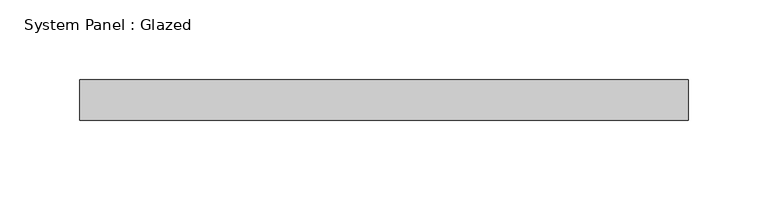
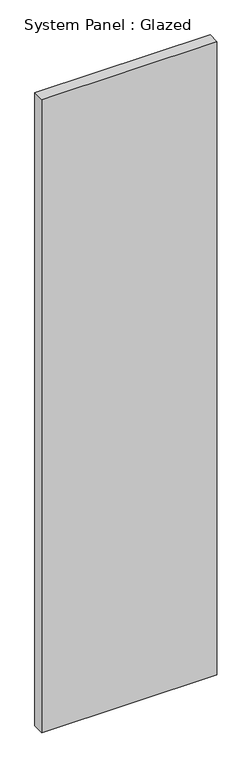
"""IFC4 building model written with IfcOpenShell, lengths in millimetres: plate geometry, System Panel : Glazed."""

from ifc_helpers import new_model, si_unit, origin, origin_with_axes, place, context, project, spatial, polyline, outline, extrude, source, transform, mapped, element, save


def system_panel_glazed_546de4f7(model_context):
    return source(origin(), model_context, "Body", "SweptSolid", [
        extrude(outline(polyline([(190.5, 19.05), (-190.5, 19.05), (-190.5, 44.45), (190.5, 44.45), (190.5, 19.05)])), origin_with_axes(), (0.0, 0.0, 1.0), 1455.9994987),
    ])


if __name__ == "__main__":
    model = new_model("IFC4")
    model_context = context("Model", 3, world=origin())
    ifc_project = project(units=[si_unit("LENGTHUNIT", "METRE", prefix="MILLI")], contexts=[model_context])
    site = spatial("IfcSite", under=ifc_project)
    building = spatial("IfcBuilding", under=site)
    placement = place(None, origin())
    system_panel_glazed_shape = system_panel_glazed_546de4f7(model_context)
    element("IfcPlate", 1, ObjectType="System Panel : Glazed", at=placement, inside=building, context=model_context, shape_type="MappedRepresentation", body=[
        mapped(system_panel_glazed_shape, transform((0.0, 0.0, 0.0), x_axis=(1.0, 0.0, 0.0), y_axis=(0.0, 1.0, 0.0), z_axis=(0.0, 0.0, 1.0))),
    ])
    save(model, "model.ifc")

# Revit data of these elements
# Type "System Panel : Glazed"
#   Construction Type Id = "GSP4R"
#   Analytic Construction = "1/8 in Pilkington single glazing"
#   Visual Light Transmittance = 0.9
#   Solar Heat Gain Coefficient = 0.86
#   Heat Transfer Coefficient (U) = 1.18115 BTU/(h·ft²·°F)
#   Define Thermal Properties by = 1
# Element 1 (IfcPlate, "System Panel : Glazed")
#   Materials on its faces: "Glass"
# Materials
#   "Glass": class "Glass", colour RGB 0 128 192, transparency 0.75, Description = "Soda Lime Glass", Cost = 0
